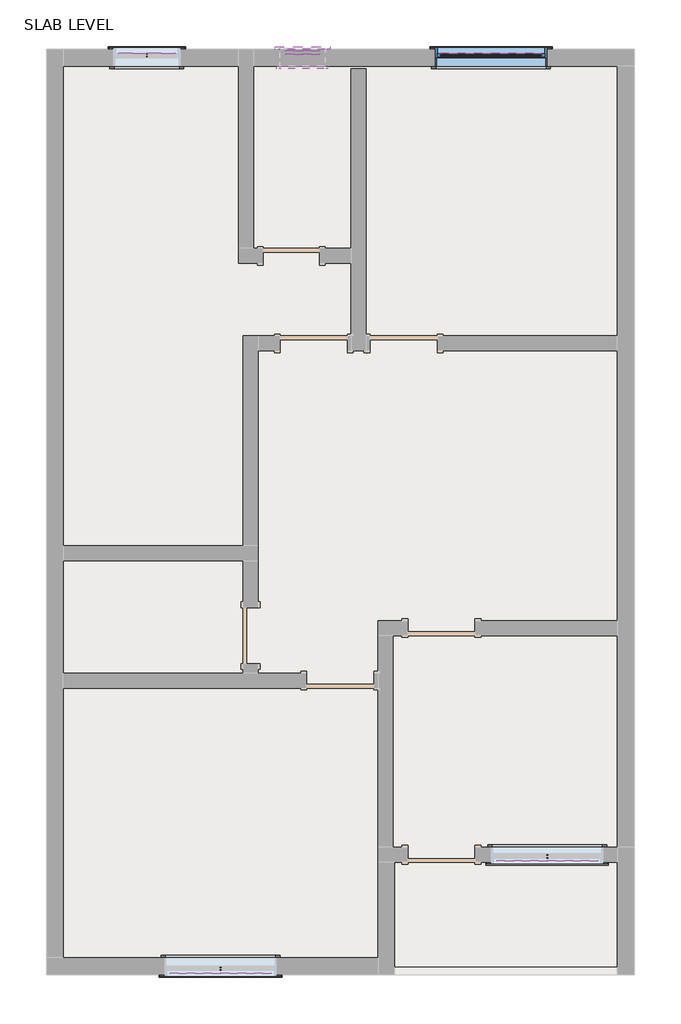
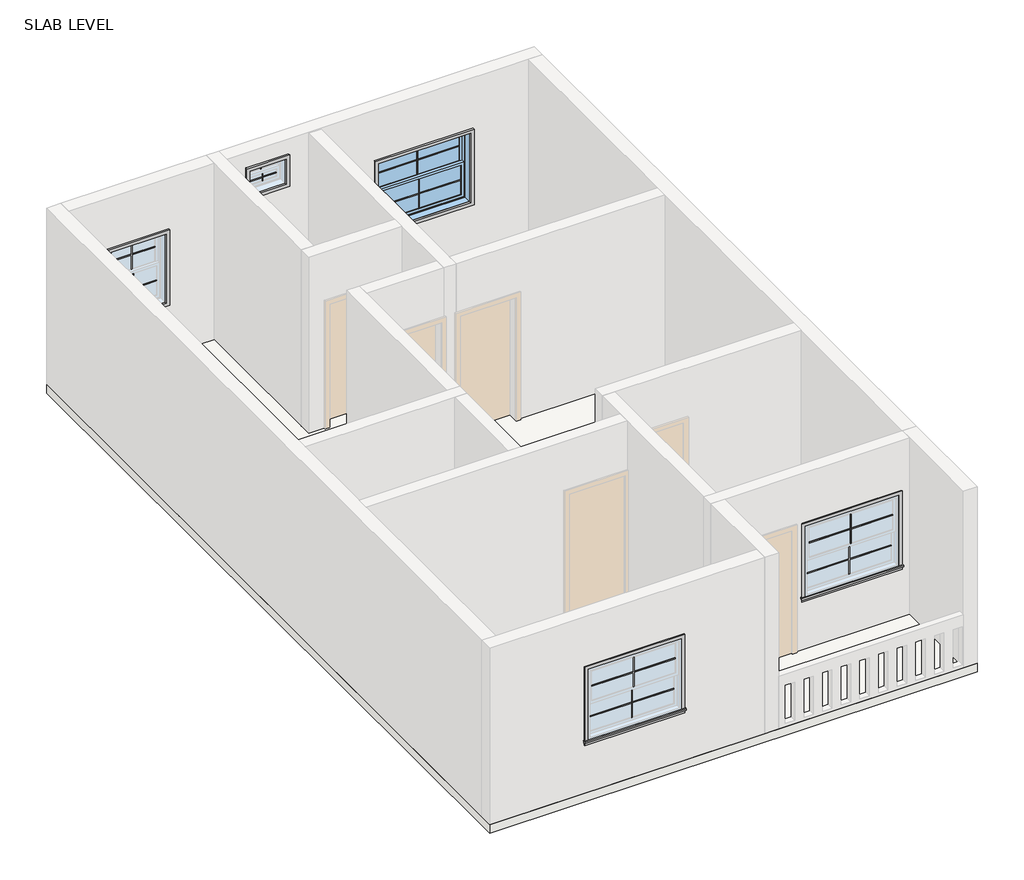
# One storey, part 2 of 2: 20 proxies, 1 railing, 1 slab, 1 window.
"""IFC4 building model written with IfcOpenShell, lengths in millimetres."""

from ifc_helpers import new_model, si_unit, frame, origin, place, context, project, spatial, polyline, outline, extrude, faceted_brep, transform, mapped, element, save
from components import muntin_pattern_2x2_muntin_pattern_2x2_c001a7f4, muntin_pattern_2x2_muntin_pattern_2x2_019d64ce, muntin_pattern_2x2_muntin_pattern_2x2_f2410a90, trim_window_exterior_flat_with_sill_7631c5ba, trim_window_exterior_flat_with_sill_f6d2a3b8, trim_window_exterior_flat_with_sill_e4b28ec3, trim_window_interior_flat_picture_frame_0f2e31f9, trim_window_interior_flat_picture_frame_f985c0ae, trim_window_interior_flat_picture_frame_39ff4276, window_a144fa31

model = new_model("IFC4")

# Units and contexts
model_context = context("Model", 3, world=origin())
ifc_project = project(units=[si_unit("LENGTHUNIT", "METRE", prefix="MILLI")], contexts=[model_context])

# Site, building, storey
site = spatial("IfcSite", under=ifc_project)
building = spatial("IfcBuilding", under=site)
storey = spatial("IfcBuildingStorey", under=building, Name="SLAB LEVEL", Elevation=3048.0)

# Proxies
placement = place(None, origin())
muntin_pattern_2x2_muntin_pattern_2x2_shape = muntin_pattern_2x2_muntin_pattern_2x2_c001a7f4(model_context)
element("IfcBuildingElementProxy", 1, Name="Muntin Pattern_2x2 : Muntin Pattern_2x2", ObjectType="Muntin Pattern_2x2 : Muntin Pattern_2x2", at=placement, inside=storey, context=model_context, shape_type="MappedRepresentation", body=[
    mapped(muntin_pattern_2x2_muntin_pattern_2x2_shape, transform((-1687.6519453, 5530.9694012, 4594.225), x_axis=(-1.0, 0.0, 0.0), y_axis=(0.0, -1.0, 0.0), z_axis=(0.0, 0.0, 1.0))),
])
element("IfcBuildingElementProxy", 2, Name="Muntin Pattern_2x2 : Muntin Pattern_2x2", ObjectType="Muntin Pattern_2x2 : Muntin Pattern_2x2", at=placement, inside=storey, context=model_context, shape_type="MappedRepresentation", body=[
    mapped(muntin_pattern_2x2_muntin_pattern_2x2_shape, transform((-1687.6519453, 5575.4194012, 4038.6), x_axis=(-1.0, 0.0, 0.0), y_axis=(0.0, -1.0, 0.0), z_axis=(0.0, 0.0, 1.0))),
])
element("IfcBuildingElementProxy", 3, Name="Muntin Pattern_2x2 : Muntin Pattern_2x2", ObjectType="Muntin Pattern_2x2 : Muntin Pattern_2x2", at=placement, inside=storey, context=model_context, shape_type="MappedRepresentation", body=[
    mapped(muntin_pattern_2x2_muntin_pattern_2x2_shape, transform((-6119.9519453, 4006.9694012, 4594.225), x_axis=(-1.0, 0.0, 0.0), y_axis=(0.0, -1.0, 0.0), z_axis=(0.0, 0.0, 1.0))),
])
element("IfcBuildingElementProxy", 4, Name="Muntin Pattern_2x2 : Muntin Pattern_2x2", ObjectType="Muntin Pattern_2x2 : Muntin Pattern_2x2", at=placement, inside=storey, context=model_context, shape_type="MappedRepresentation", body=[
    mapped(muntin_pattern_2x2_muntin_pattern_2x2_shape, transform((-6119.9519453, 4051.4194012, 4038.6), x_axis=(-1.0, 0.0, 0.0), y_axis=(0.0, -1.0, 0.0), z_axis=(0.0, 0.0, 1.0))),
])
element("IfcBuildingElementProxy", 5, Name="Muntin Pattern_2x2 : Muntin Pattern_2x2", ObjectType="Muntin Pattern_2x2 : Muntin Pattern_2x2", at=placement, inside=storey, context=model_context, shape_type="MappedRepresentation", body=[
    mapped(muntin_pattern_2x2_muntin_pattern_2x2_shape, transform((-2449.6519453, 16484.7194012, 4594.225), x_axis=(1.0, 0.0, 0.0), y_axis=(0.0, 1.0, 0.0), z_axis=(0.0, 0.0, 1.0))),
])
element("IfcBuildingElementProxy", 6, Name="Muntin Pattern_2x2 : Muntin Pattern_2x2", ObjectType="Muntin Pattern_2x2 : Muntin Pattern_2x2", at=placement, inside=storey, context=model_context, shape_type="MappedRepresentation", body=[
    mapped(muntin_pattern_2x2_muntin_pattern_2x2_shape, transform((-2449.6519453, 16440.2694012, 4038.6), x_axis=(1.0, 0.0, 0.0), y_axis=(0.0, 1.0, 0.0), z_axis=(0.0, 0.0, 1.0))),
])
muntin_pattern_2x2_muntin_pattern_2x2_2_shape = muntin_pattern_2x2_muntin_pattern_2x2_019d64ce(model_context)
element("IfcBuildingElementProxy", 7, Name="Muntin Pattern_2x2 : Muntin Pattern_2x2", ObjectType="Muntin Pattern_2x2 : Muntin Pattern_2x2", at=placement, inside=storey, context=model_context, shape_type="MappedRepresentation", body=[
    mapped(muntin_pattern_2x2_muntin_pattern_2x2_2_shape, transform((-5008.7019453, 16484.7194012, 5584.825), x_axis=(1.0, 0.0, 0.0), y_axis=(0.0, 1.0, 0.0), z_axis=(0.0, 0.0, 1.0))),
])
element("IfcBuildingElementProxy", 8, Name="Muntin Pattern_2x2 : Muntin Pattern_2x2", ObjectType="Muntin Pattern_2x2 : Muntin Pattern_2x2", at=placement, inside=storey, context=model_context, shape_type="MappedRepresentation", body=[
    mapped(muntin_pattern_2x2_muntin_pattern_2x2_2_shape, transform((-5008.7019453, 16440.2694012, 5410.2), x_axis=(1.0, 0.0, 0.0), y_axis=(0.0, 1.0, 0.0), z_axis=(0.0, 0.0, 1.0))),
])
muntin_pattern_2x2_muntin_pattern_2x2_3_shape = muntin_pattern_2x2_muntin_pattern_2x2_f2410a90(model_context)
element("IfcBuildingElementProxy", 9, Name="Muntin Pattern_2x2 : Muntin Pattern_2x2", ObjectType="Muntin Pattern_2x2 : Muntin Pattern_2x2", at=placement, inside=storey, context=model_context, shape_type="MappedRepresentation", body=[
    mapped(muntin_pattern_2x2_muntin_pattern_2x2_3_shape, transform((-7120.0769453, 16484.7194012, 4594.225), x_axis=(1.0, 0.0, 0.0), y_axis=(0.0, 1.0, 0.0), z_axis=(0.0, 0.0, 1.0))),
])
element("IfcBuildingElementProxy", 10, Name="Muntin Pattern_2x2 : Muntin Pattern_2x2", ObjectType="Muntin Pattern_2x2 : Muntin Pattern_2x2", at=placement, inside=storey, context=model_context, shape_type="MappedRepresentation", body=[
    mapped(muntin_pattern_2x2_muntin_pattern_2x2_3_shape, transform((-7120.0769453, 16440.2694012, 4038.6), x_axis=(1.0, 0.0, 0.0), y_axis=(0.0, 1.0, 0.0), z_axis=(0.0, 0.0, 1.0))),
])
trim_window_exterior_flat_with_sill_shape = trim_window_exterior_flat_with_sill_7631c5ba(model_context)
element("IfcBuildingElementProxy", 11, Name="Trim-Window-Exterior-Flat : with Sill", ObjectType="Trim-Window-Exterior-Flat : with Sill", at=placement, inside=storey, context=model_context, shape_type="MappedRepresentation", body=[
    mapped(trim_window_exterior_flat_with_sill_shape, transform((-1687.6519453, 5496.0444012, 5181.6), x_axis=(1.0, 0.0, 0.0), y_axis=(0.0, 0.0, 1.0), z_axis=(0.0, -1.0, 0.0))),
])
element("IfcBuildingElementProxy", 12, Name="Trim-Window-Exterior-Flat : with Sill", ObjectType="Trim-Window-Exterior-Flat : with Sill", at=placement, inside=storey, context=model_context, shape_type="MappedRepresentation", body=[
    mapped(trim_window_exterior_flat_with_sill_shape, transform((-6119.9519453, 3972.0444012, 5181.6), x_axis=(1.0, 0.0, 0.0), y_axis=(0.0, 0.0, 1.0), z_axis=(0.0, -1.0, 0.0))),
])
element("IfcBuildingElementProxy", 13, Name="Trim-Window-Exterior-Flat : with Sill", ObjectType="Trim-Window-Exterior-Flat : with Sill", at=placement, inside=storey, context=model_context, shape_type="MappedRepresentation", body=[
    mapped(trim_window_exterior_flat_with_sill_shape, transform((-2449.6519453, 16519.6444012, 5181.6), x_axis=(-1.0, 0.0, 0.0), y_axis=(0.0, 0.0, 1.0), z_axis=(0.0, 1.0, 0.0))),
])
trim_window_exterior_flat_with_sill_2_shape = trim_window_exterior_flat_with_sill_f6d2a3b8(model_context)
element("IfcBuildingElementProxy", 14, Name="Trim-Window-Exterior-Flat : with Sill", ObjectType="Trim-Window-Exterior-Flat : with Sill", at=placement, inside=storey, context=model_context, shape_type="MappedRepresentation", body=[
    mapped(trim_window_exterior_flat_with_sill_2_shape, transform((-5008.7019453, 16519.6444012, 5791.2), x_axis=(-1.0, 0.0, 0.0), y_axis=(0.0, 0.0, 1.0), z_axis=(0.0, 1.0, 0.0))),
])
trim_window_exterior_flat_with_sill_3_shape = trim_window_exterior_flat_with_sill_e4b28ec3(model_context)
element("IfcBuildingElementProxy", 15, Name="Trim-Window-Exterior-Flat : with Sill", ObjectType="Trim-Window-Exterior-Flat : with Sill", at=placement, inside=storey, context=model_context, shape_type="MappedRepresentation", body=[
    mapped(trim_window_exterior_flat_with_sill_3_shape, transform((-7120.0769453, 16519.6444012, 5181.6), x_axis=(-1.0, 0.0, 0.0), y_axis=(0.0, 0.0, 1.0), z_axis=(0.0, 1.0, 0.0))),
])
trim_window_interior_flat_picture_frame_shape = trim_window_interior_flat_picture_frame_0f2e31f9(model_context)
element("IfcBuildingElementProxy", 16, Name="Trim-Window-Interior-Flat : Picture Frame", ObjectType="Trim-Window-Interior-Flat : Picture Frame", at=placement, inside=storey, context=model_context, shape_type="MappedRepresentation", body=[
    mapped(trim_window_interior_flat_picture_frame_shape, transform((-1687.6519453, 5699.2444012, 5181.6), x_axis=(-1.0, 0.0, 0.0), y_axis=(0.0, 0.0, 1.0), z_axis=(0.0, 1.0, 0.0))),
])
element("IfcBuildingElementProxy", 17, Name="Trim-Window-Interior-Flat : Picture Frame", ObjectType="Trim-Window-Interior-Flat : Picture Frame", at=placement, inside=storey, context=model_context, shape_type="MappedRepresentation", body=[
    mapped(trim_window_interior_flat_picture_frame_shape, transform((-6119.9519453, 4200.6444012, 5181.6), x_axis=(-1.0, 0.0, 0.0), y_axis=(0.0, 0.0, 1.0), z_axis=(0.0, 1.0, 0.0))),
])
element("IfcBuildingElementProxy", 18, Name="Trim-Window-Interior-Flat : Picture Frame", ObjectType="Trim-Window-Interior-Flat : Picture Frame", at=placement, inside=storey, context=model_context, shape_type="MappedRepresentation", body=[
    mapped(trim_window_interior_flat_picture_frame_shape, transform((-2449.6519453, 16291.0444012, 5181.6), x_axis=(1.0, 0.0, 0.0), y_axis=(0.0, 0.0, 1.0), z_axis=(0.0, -1.0, 0.0))),
])
trim_window_interior_flat_picture_frame_2_shape = trim_window_interior_flat_picture_frame_f985c0ae(model_context)
element("IfcBuildingElementProxy", 19, Name="Trim-Window-Interior-Flat : Picture Frame", ObjectType="Trim-Window-Interior-Flat : Picture Frame", at=placement, inside=storey, context=model_context, shape_type="MappedRepresentation", body=[
    mapped(trim_window_interior_flat_picture_frame_2_shape, transform((-5008.7019453, 16291.0444012, 5791.2), x_axis=(1.0, 0.0, 0.0), y_axis=(0.0, 0.0, 1.0), z_axis=(0.0, -1.0, 0.0))),
])
trim_window_interior_flat_picture_frame_3_shape = trim_window_interior_flat_picture_frame_39ff4276(model_context)
element("IfcBuildingElementProxy", 20, Name="Trim-Window-Interior-Flat : Picture Frame", ObjectType="Trim-Window-Interior-Flat : Picture Frame", at=placement, inside=storey, context=model_context, shape_type="MappedRepresentation", body=[
    mapped(trim_window_interior_flat_picture_frame_3_shape, transform((-7120.0769453, 16291.0444012, 5181.6), x_axis=(1.0, 0.0, 0.0), y_axis=(0.0, 0.0, 1.0), z_axis=(0.0, -1.0, 0.0))),
])

# Railing
element("IfcRailing", 21, ObjectType="Handrail - Rectangular", at=placement, inside=storey, context=model_context, shape_type="SolidModel", body=[
    faceted_brep([(-3275.1519453, 16430.7444012, 1828.8), (-3275.1519453, 16430.7444012, 1778.0), (-3275.1519453, 16379.9444012, 1778.0), (-3275.1519453, 16379.9444012, 1828.8), (-595.4519453, 16430.7444012, 1828.8), (-595.4519453, 16430.7444012, 1778.0), (-646.2519453, 16379.9444012, 1778.0), (-646.2519453, 16379.9444012, 1828.8), (-595.4519453, 14970.2444012, 1828.8), (-646.2519453, 14970.2444012, 1828.8), (-646.2519453, 14970.2444012, 1778.0), (-595.4519453, 14970.2444012, 1778.0)], [[[0, 1, 2, 3]], [[1, 0, 4, 5]], [[2, 1, 5, 6]], [[3, 2, 6, 7]], [[0, 3, 7, 4]], [[8, 9, 10, 11]], [[5, 4, 8, 11]], [[6, 5, 11, 10]], [[7, 6, 10, 9]], [[4, 7, 9, 8]]]),
    extrude(outline(polyline([(-630.3769453, 14992.4694012), (-611.3269453, 14992.4694012), (-611.3269453, 14973.4194012), (-630.3769453, 14973.4194012), (-630.3769453, 14992.4694012)])), frame((0.0, 0.0, 914.4), z_axis=(0.0, 0.0, 1.0), x_axis=(1.0, 0.0, 0.0)), (0.0, 0.0, 1.0), 863.6),
    extrude(outline(polyline([(-630.3769453, 15094.0694012), (-611.3269453, 15094.0694012), (-611.3269453, 15075.0194012), (-630.3769453, 15075.0194012), (-630.3769453, 15094.0694012)])), frame((0.0, 0.0, 914.4), z_axis=(0.0, 0.0, 1.0), x_axis=(1.0, 0.0, 0.0)), (0.0, 0.0, 1.0), 863.6),
    extrude(outline(polyline([(-630.3769453, 15195.6694012), (-611.3269453, 15195.6694012), (-611.3269453, 15176.6194012), (-630.3769453, 15176.6194012), (-630.3769453, 15195.6694012)])), frame((0.0, 0.0, 914.4), z_axis=(0.0, 0.0, 1.0), x_axis=(1.0, 0.0, 0.0)), (0.0, 0.0, 1.0), 863.6),
    extrude(outline(polyline([(-630.3769453, 15297.2694012), (-611.3269453, 15297.2694012), (-611.3269453, 15278.2194012), (-630.3769453, 15278.2194012), (-630.3769453, 15297.2694012)])), frame((0.0, 0.0, 914.4), z_axis=(0.0, 0.0, 1.0), x_axis=(1.0, 0.0, 0.0)), (0.0, 0.0, 1.0), 863.6),
    extrude(outline(polyline([(-630.3769453, 15398.8694012), (-611.3269453, 15398.8694012), (-611.3269453, 15379.8194012), (-630.3769453, 15379.8194012), (-630.3769453, 15398.8694012)])), frame((0.0, 0.0, 914.4), z_axis=(0.0, 0.0, 1.0), x_axis=(1.0, 0.0, 0.0)), (0.0, 0.0, 1.0), 863.6),
    extrude(outline(polyline([(-630.3769453, 15500.4694012), (-611.3269453, 15500.4694012), (-611.3269453, 15481.4194012), (-630.3769453, 15481.4194012), (-630.3769453, 15500.4694012)])), frame((0.0, 0.0, 914.4), z_axis=(0.0, 0.0, 1.0), x_axis=(1.0, 0.0, 0.0)), (0.0, 0.0, 1.0), 863.6),
    extrude(outline(polyline([(-630.3769453, 15602.0694012), (-611.3269453, 15602.0694012), (-611.3269453, 15583.0194012), (-630.3769453, 15583.0194012), (-630.3769453, 15602.0694012)])), frame((0.0, 0.0, 914.4), z_axis=(0.0, 0.0, 1.0), x_axis=(1.0, 0.0, 0.0)), (0.0, 0.0, 1.0), 863.6),
    extrude(outline(polyline([(-630.3769453, 15703.6694012), (-611.3269453, 15703.6694012), (-611.3269453, 15684.6194012), (-630.3769453, 15684.6194012), (-630.3769453, 15703.6694012)])), frame((0.0, 0.0, 914.4), z_axis=(0.0, 0.0, 1.0), x_axis=(1.0, 0.0, 0.0)), (0.0, 0.0, 1.0), 863.6),
    extrude(outline(polyline([(-630.3769453, 15805.2694012), (-611.3269453, 15805.2694012), (-611.3269453, 15786.2194012), (-630.3769453, 15786.2194012), (-630.3769453, 15805.2694012)])), frame((0.0, 0.0, 914.4), z_axis=(0.0, 0.0, 1.0), x_axis=(1.0, 0.0, 0.0)), (0.0, 0.0, 1.0), 863.6),
    extrude(outline(polyline([(-630.3769453, 15906.8694012), (-611.3269453, 15906.8694012), (-611.3269453, 15887.8194012), (-630.3769453, 15887.8194012), (-630.3769453, 15906.8694012)])), frame((0.0, 0.0, 914.4), z_axis=(0.0, 0.0, 1.0), x_axis=(1.0, 0.0, 0.0)), (0.0, 0.0, 1.0), 863.6),
    extrude(outline(polyline([(-630.3769453, 16008.4694012), (-611.3269453, 16008.4694012), (-611.3269453, 15989.4194012), (-630.3769453, 15989.4194012), (-630.3769453, 16008.4694012)])), frame((0.0, 0.0, 914.4), z_axis=(0.0, 0.0, 1.0), x_axis=(1.0, 0.0, 0.0)), (0.0, 0.0, 1.0), 863.6),
    extrude(outline(polyline([(-630.3769453, 16110.0694012), (-611.3269453, 16110.0694012), (-611.3269453, 16091.0194012), (-630.3769453, 16091.0194012), (-630.3769453, 16110.0694012)])), frame((0.0, 0.0, 914.4), z_axis=(0.0, 0.0, 1.0), x_axis=(1.0, 0.0, 0.0)), (0.0, 0.0, 1.0), 863.6),
    extrude(outline(polyline([(-630.3769453, 16211.6694012), (-611.3269453, 16211.6694012), (-611.3269453, 16192.6194012), (-630.3769453, 16192.6194012), (-630.3769453, 16211.6694012)])), frame((0.0, 0.0, 914.4), z_axis=(0.0, 0.0, 1.0), x_axis=(1.0, 0.0, 0.0)), (0.0, 0.0, 1.0), 863.6),
    extrude(outline(polyline([(-630.3769453, 16313.2694012), (-611.3269453, 16313.2694012), (-611.3269453, 16294.2194012), (-630.3769453, 16294.2194012), (-630.3769453, 16313.2694012)])), frame((0.0, 0.0, 914.4), z_axis=(0.0, 0.0, 1.0), x_axis=(1.0, 0.0, 0.0)), (0.0, 0.0, 1.0), 863.6),
    extrude(outline(polyline([(-643.0769453, 16395.8194012), (-643.0769453, 16414.8694012), (-624.0269453, 16414.8694012), (-624.0269453, 16395.8194012), (-643.0769453, 16395.8194012)])), frame((0.0, 0.0, 914.4), z_axis=(0.0, 0.0, 1.0), x_axis=(1.0, 0.0, 0.0)), (0.0, 0.0, 1.0), 863.6),
    extrude(outline(polyline([(-744.6769453, 16395.8194012), (-744.6769453, 16414.8694012), (-725.6269453, 16414.8694012), (-725.6269453, 16395.8194012), (-744.6769453, 16395.8194012)])), frame((0.0, 0.0, 914.4), z_axis=(0.0, 0.0, 1.0), x_axis=(1.0, 0.0, 0.0)), (0.0, 0.0, 1.0), 863.6),
    extrude(outline(polyline([(-846.2769453, 16395.8194012), (-846.2769453, 16414.8694012), (-827.2269453, 16414.8694012), (-827.2269453, 16395.8194012), (-846.2769453, 16395.8194012)])), frame((0.0, 0.0, 914.4), z_axis=(0.0, 0.0, 1.0), x_axis=(1.0, 0.0, 0.0)), (0.0, 0.0, 1.0), 863.6),
    extrude(outline(polyline([(-947.8769453, 16395.8194012), (-947.8769453, 16414.8694012), (-928.8269453, 16414.8694012), (-928.8269453, 16395.8194012), (-947.8769453, 16395.8194012)])), frame((0.0, 0.0, 914.4), z_axis=(0.0, 0.0, 1.0), x_axis=(1.0, 0.0, 0.0)), (0.0, 0.0, 1.0), 863.6),
    extrude(outline(polyline([(-1049.4769453, 16395.8194012), (-1049.4769453, 16414.8694012), (-1030.4269453, 16414.8694012), (-1030.4269453, 16395.8194012), (-1049.4769453, 16395.8194012)])), frame((0.0, 0.0, 914.4), z_axis=(0.0, 0.0, 1.0), x_axis=(1.0, 0.0, 0.0)), (0.0, 0.0, 1.0), 863.6),
    extrude(outline(polyline([(-1151.0769453, 16395.8194012), (-1151.0769453, 16414.8694012), (-1132.0269453, 16414.8694012), (-1132.0269453, 16395.8194012), (-1151.0769453, 16395.8194012)])), frame((0.0, 0.0, 914.4), z_axis=(0.0, 0.0, 1.0), x_axis=(1.0, 0.0, 0.0)), (0.0, 0.0, 1.0), 863.6),
    extrude(outline(polyline([(-1252.6769453, 16395.8194012), (-1252.6769453, 16414.8694012), (-1233.6269453, 16414.8694012), (-1233.6269453, 16395.8194012), (-1252.6769453, 16395.8194012)])), frame((0.0, 0.0, 914.4), z_axis=(0.0, 0.0, 1.0), x_axis=(1.0, 0.0, 0.0)), (0.0, 0.0, 1.0), 863.6),
    extrude(outline(polyline([(-1354.2769453, 16395.8194012), (-1354.2769453, 16414.8694012), (-1335.2269453, 16414.8694012), (-1335.2269453, 16395.8194012), (-1354.2769453, 16395.8194012)])), frame((0.0, 0.0, 914.4), z_axis=(0.0, 0.0, 1.0), x_axis=(1.0, 0.0, 0.0)), (0.0, 0.0, 1.0), 863.6),
    extrude(outline(polyline([(-1455.8769453, 16395.8194012), (-1455.8769453, 16414.8694012), (-1436.8269453, 16414.8694012), (-1436.8269453, 16395.8194012), (-1455.8769453, 16395.8194012)])), frame((0.0, 0.0, 914.4), z_axis=(0.0, 0.0, 1.0), x_axis=(1.0, 0.0, 0.0)), (0.0, 0.0, 1.0), 863.6),
    extrude(outline(polyline([(-1557.4769453, 16395.8194012), (-1557.4769453, 16414.8694012), (-1538.4269453, 16414.8694012), (-1538.4269453, 16395.8194012), (-1557.4769453, 16395.8194012)])), frame((0.0, 0.0, 914.4), z_axis=(0.0, 0.0, 1.0), x_axis=(1.0, 0.0, 0.0)), (0.0, 0.0, 1.0), 863.6),
    extrude(outline(polyline([(-1659.0769453, 16395.8194012), (-1659.0769453, 16414.8694012), (-1640.0269453, 16414.8694012), (-1640.0269453, 16395.8194012), (-1659.0769453, 16395.8194012)])), frame((0.0, 0.0, 914.4), z_axis=(0.0, 0.0, 1.0), x_axis=(1.0, 0.0, 0.0)), (0.0, 0.0, 1.0), 863.6),
    extrude(outline(polyline([(-1760.6769453, 16395.8194012), (-1760.6769453, 16414.8694012), (-1741.6269453, 16414.8694012), (-1741.6269453, 16395.8194012), (-1760.6769453, 16395.8194012)])), frame((0.0, 0.0, 914.4), z_axis=(0.0, 0.0, 1.0), x_axis=(1.0, 0.0, 0.0)), (0.0, 0.0, 1.0), 863.6),
    extrude(outline(polyline([(-1862.2769453, 16395.8194012), (-1862.2769453, 16414.8694012), (-1843.2269453, 16414.8694012), (-1843.2269453, 16395.8194012), (-1862.2769453, 16395.8194012)])), frame((0.0, 0.0, 914.4), z_axis=(0.0, 0.0, 1.0), x_axis=(1.0, 0.0, 0.0)), (0.0, 0.0, 1.0), 863.6),
    extrude(outline(polyline([(-1963.8769453, 16395.8194012), (-1963.8769453, 16414.8694012), (-1944.8269453, 16414.8694012), (-1944.8269453, 16395.8194012), (-1963.8769453, 16395.8194012)])), frame((0.0, 0.0, 914.4), z_axis=(0.0, 0.0, 1.0), x_axis=(1.0, 0.0, 0.0)), (0.0, 0.0, 1.0), 863.6),
    extrude(outline(polyline([(-2065.4769453, 16395.8194012), (-2065.4769453, 16414.8694012), (-2046.4269453, 16414.8694012), (-2046.4269453, 16395.8194012), (-2065.4769453, 16395.8194012)])), frame((0.0, 0.0, 914.4), z_axis=(0.0, 0.0, 1.0), x_axis=(1.0, 0.0, 0.0)), (0.0, 0.0, 1.0), 863.6),
    extrude(outline(polyline([(-2167.0769453, 16395.8194012), (-2167.0769453, 16414.8694012), (-2148.0269453, 16414.8694012), (-2148.0269453, 16395.8194012), (-2167.0769453, 16395.8194012)])), frame((0.0, 0.0, 914.4), z_axis=(0.0, 0.0, 1.0), x_axis=(1.0, 0.0, 0.0)), (0.0, 0.0, 1.0), 863.6),
    extrude(outline(polyline([(-2268.6769453, 16395.8194012), (-2268.6769453, 16414.8694012), (-2249.6269453, 16414.8694012), (-2249.6269453, 16395.8194012), (-2268.6769453, 16395.8194012)])), frame((0.0, 0.0, 914.4), z_axis=(0.0, 0.0, 1.0), x_axis=(1.0, 0.0, 0.0)), (0.0, 0.0, 1.0), 863.6),
    extrude(outline(polyline([(-2370.2769453, 16395.8194012), (-2370.2769453, 16414.8694012), (-2351.2269453, 16414.8694012), (-2351.2269453, 16395.8194012), (-2370.2769453, 16395.8194012)])), frame((0.0, 0.0, 914.4), z_axis=(0.0, 0.0, 1.0), x_axis=(1.0, 0.0, 0.0)), (0.0, 0.0, 1.0), 863.6),
    extrude(outline(polyline([(-2471.8769453, 16395.8194012), (-2471.8769453, 16414.8694012), (-2452.8269453, 16414.8694012), (-2452.8269453, 16395.8194012), (-2471.8769453, 16395.8194012)])), frame((0.0, 0.0, 914.4), z_axis=(0.0, 0.0, 1.0), x_axis=(1.0, 0.0, 0.0)), (0.0, 0.0, 1.0), 863.6),
    extrude(outline(polyline([(-2573.4769453, 16395.8194012), (-2573.4769453, 16414.8694012), (-2554.4269453, 16414.8694012), (-2554.4269453, 16395.8194012), (-2573.4769453, 16395.8194012)])), frame((0.0, 0.0, 914.4), z_axis=(0.0, 0.0, 1.0), x_axis=(1.0, 0.0, 0.0)), (0.0, 0.0, 1.0), 863.6),
    extrude(outline(polyline([(-2675.0769453, 16395.8194012), (-2675.0769453, 16414.8694012), (-2656.0269453, 16414.8694012), (-2656.0269453, 16395.8194012), (-2675.0769453, 16395.8194012)])), frame((0.0, 0.0, 914.4), z_axis=(0.0, 0.0, 1.0), x_axis=(1.0, 0.0, 0.0)), (0.0, 0.0, 1.0), 863.6),
    extrude(outline(polyline([(-2776.6769453, 16395.8194012), (-2776.6769453, 16414.8694012), (-2757.6269453, 16414.8694012), (-2757.6269453, 16395.8194012), (-2776.6769453, 16395.8194012)])), frame((0.0, 0.0, 914.4), z_axis=(0.0, 0.0, 1.0), x_axis=(1.0, 0.0, 0.0)), (0.0, 0.0, 1.0), 863.6),
    extrude(outline(polyline([(-2878.2769453, 16395.8194012), (-2878.2769453, 16414.8694012), (-2859.2269453, 16414.8694012), (-2859.2269453, 16395.8194012), (-2878.2769453, 16395.8194012)])), frame((0.0, 0.0, 914.4), z_axis=(0.0, 0.0, 1.0), x_axis=(1.0, 0.0, 0.0)), (0.0, 0.0, 1.0), 863.6),
    extrude(outline(polyline([(-2979.8769453, 16395.8194012), (-2979.8769453, 16414.8694012), (-2960.8269453, 16414.8694012), (-2960.8269453, 16395.8194012), (-2979.8769453, 16395.8194012)])), frame((0.0, 0.0, 914.4), z_axis=(0.0, 0.0, 1.0), x_axis=(1.0, 0.0, 0.0)), (0.0, 0.0, 1.0), 863.6),
    extrude(outline(polyline([(-3081.4769453, 16395.8194012), (-3081.4769453, 16414.8694012), (-3062.4269453, 16414.8694012), (-3062.4269453, 16395.8194012), (-3081.4769453, 16395.8194012)])), frame((0.0, 0.0, 914.4), z_axis=(0.0, 0.0, 1.0), x_axis=(1.0, 0.0, 0.0)), (0.0, 0.0, 1.0), 863.6),
    extrude(outline(polyline([(-3183.0769453, 16395.8194012), (-3183.0769453, 16414.8694012), (-3164.0269453, 16414.8694012), (-3164.0269453, 16395.8194012), (-3183.0769453, 16395.8194012)])), frame((0.0, 0.0, 914.4), z_axis=(0.0, 0.0, 1.0), x_axis=(1.0, 0.0, 0.0)), (0.0, 0.0, 1.0), 863.6),
    extrude(outline(polyline([(-630.3769453, 16395.8194012), (-630.3769453, 16414.8694012), (-611.3269453, 16414.8694012), (-611.3269453, 16395.8194012), (-630.3769453, 16395.8194012)])), frame((0.0, 0.0, 914.4), z_axis=(0.0, 0.0, 1.0), x_axis=(1.0, 0.0, 0.0)), (0.0, 0.0, 1.0), 863.6),
    extrude(outline(polyline([(-630.3769453, 14989.2944012), (-611.3269453, 14989.2944012), (-611.3269453, 14970.2444012), (-630.3769453, 14970.2444012), (-630.3769453, 14989.2944012)])), frame((0.0, 0.0, 914.4), z_axis=(0.0, 0.0, 1.0), x_axis=(1.0, 0.0, 0.0)), (0.0, 0.0, 1.0), 863.6),
    extrude(outline(polyline([(-3275.1519453, 16395.8194012), (-3275.1519453, 16414.8694012), (-3256.1019453, 16414.8694012), (-3256.1019453, 16395.8194012), (-3275.1519453, 16395.8194012)])), frame((0.0, 0.0, 914.4), z_axis=(0.0, 0.0, 1.0), x_axis=(1.0, 0.0, 0.0)), (0.0, 0.0, 1.0), 863.6),
])

# Slab
element("IfcSlab", 22, ObjectType="SLAB 6\"", at=placement, inside=storey, context=model_context, shape_type="SweptSolid", body=[
    extrude(outline(polyline([(-506.5519453, 3972.0444012), (-8482.1519453, 3972.0444012), (-8482.1519453, 16519.6444012), (-506.5519453, 16519.6444012), (-506.5519453, 3972.0444012)])), frame((0.0, 0.0, 2895.6), z_axis=(0.0, 0.0, 1.0), x_axis=(1.0, 0.0, 0.0)), (0.0, 0.0, 1.0), 152.4),
])

# Window
window_shape = window_a144fa31(model_context)
element("IfcWindow", 23, ObjectType="Window-Double-Hung : 60\"X48\"", at=placement, inside=storey, context=model_context, shape_type="MappedRepresentation", body=[
    mapped(window_shape, transform((-2449.6519453, 16405.3444012, 3048.0), x_axis=(1.0, 0.0, 0.0), y_axis=(0.0, 1.0, 0.0), z_axis=(0.0, 0.0, 1.0))),
])

save(model, "model.ifc")

# Revit data of these elements
# Type "Muntin Pattern_2x2 : Muntin Pattern_2x2"
#   Width [instance default] = 4' - 0"
#   Thickness = 0' - 0 1/2"
#   Height [instance default] = 4' - 0"
#   Distance = 0' - 0 3/4"
#   Interior Material [instance default] = none
#   Exterior Material [instance default] = none
#   Default Elevation = 0
# Type "Trim-Window-Exterior-Flat : with Sill"
#   Trim Width = 0' - 2 1/4"
#   Trim Thickness_Picture Frame = 0' - 1 1/4"
#   Trim Thickness_with Sill = 0' - 0 3/4"
#   Sill Thickness = 0' - 1 1/4"
#   Opening Width [instance default] = 2' - 0"
#   Opening Height [instance default] = 3' - 0"
#   Default Elevation = 4' - 0"
#   Sill = yes
#   Picture Frame = no
#   Trim Material [instance default] = none
# Type "Trim-Window-Interior-Flat : Picture Frame"
#   Trim Thickness_Picture Frame = 0' - 1 1/4"
#   Trim Width = 0' - 2 1/4"
#   Trim Thickness_with Sill = 0' - 0 3/4"
#   Sill Thickness = 0' - 1 1/4"
#   Opening Width [instance default] = 2' - 0"
#   Opening Height [instance default] = 3' - 0"
#   Default Elevation = 4' - 0"
#   Sill = no
#   Picture Frame = yes
#   Trim Material [instance default] = none
# Type "Handrail - Rectangular"
#   Assembly Code = "C2010400"
#   built-in parameter 1008612 = 0.0416667 (stored number, unit not read)
#   built-in parameter 1008611 = 0.0416667 (stored number, unit not read)
#   built-in parameter 1008609 = 0.333333 (stored number, unit not read)
#   built-in parameter 1008604 = 0.166667 (stored number, unit not read)
#   built-in parameter 1008603 = 0.166667 (stored number, unit not read)
#   Railing Height = 3' - 0"
#   built-in parameter 1008630 = 2
#   built-in parameter 1008610 = 2
#   built-in parameter 1008618 = Baluster - Square : 3/4"
# Type "SLAB 6\""
#   Assembly Code = "B1010"
#   Function = 0
#   Layers, outside or top first: 0' - 6" no material (function 1)
# Type "Window-Double-Hung : 60\"X48\""
#   Type Mark = "18"
#   Fire Rating = "0.5h"
#   Construction Type Id = "DG-DR"
#   Assembly Code = "B2020100"
#   Analytic Construction = "Double glazing - domestic"
#   Wall Thickness [instance default] = 0' - 6"
#   Window Inset [instance default] = 0' - 0"
#   Visual Light Transmittance = 0.81
#   Thermal Resistance (R) = 1.8146 (h·ft²·°F)/BTU
#   Solar Heat Gain Coefficient = 0.76
#   Muntin Width = 4' - 6"
#   Muntin Height = 1' - 8 1/8"
#   Interior Wall Closure [instance default] = 0' - 1 1/2"
#   Rough Width = 5' - 0 1/2"
#   Rough Height = 4' - 0 1/2"
#   Frame Extension [instance default] = 0' - 1 1/4"
#   Exterior Wall Closure [instance default] = 0' - 0 1/2"
#   Extension Jamb [instance default] = 0' - 1 1/2"
#   Heat Transfer Coefficient (U) = 0.5511 BTU/(h·ft²·°F)
#   Height = 4' - 0"
#   Width = 5' - 0"
#   Top Muntin Visibility = yes
#   Indicator Visibility [instance default] = yes
#   Extension Jamb Visibility [instance default] = yes
#   Interior Trim Visibility [instance default] = yes
#   Exterior Trim Visibility [instance default] = yes
#   Define Thermal Properties by = 1
#   Bottom Muntin Visibility = yes
#   Muntin Pattern = Muntin Pattern_2x2 : Muntin Pattern_2x2
#   Interior Trim Material = Wood - Stained
#   Interior Trim = Trim-Window-Interior-Flat : Picture Frame
#   Exterior Trim Material = Clad - White
#   Exterior Trim = Trim-Window-Exterior-Flat : with Sill
#   Glass Panel Material = Glass
#   Exterior Frame Material = Clad - White
#   Interior Frame Material = Wood - Stained
#   Wall Closure = (empty or 0)
# Elements 1, 2, 3, 4, 5, 6 (IfcBuildingElementProxy, "Muntin Pattern_2x2 : Muntin Pattern_2x2")
#   Width = 4' - 6"
#   Height = 1' - 8 1/8"
#   Interior Material = Wood - Stained
#   Exterior Material = Clad - White
#   Phase Created = New Construction
#   Materials on its faces: "Clad - White", "Wood - Stained"
# Elements 7, 8 (IfcBuildingElementProxy, "Muntin Pattern_2x2 : Muntin Pattern_2x2")
#   Width = 1' - 6"
#   Height = 0' - 5 1/8"
#   Interior Material = Wood - Stained
#   Exterior Material = Clad - White
#   Phase Created = New Construction
#   Materials on its faces: "Clad - White", "Wood - Stained"
# Elements 9, 10 (IfcBuildingElementProxy, "Muntin Pattern_2x2 : Muntin Pattern_2x2")
#   Width = 2' - 6"
#   Height = 1' - 8 1/8"
#   Interior Material = Wood - Stained
#   Exterior Material = Clad - White
#   Phase Created = New Construction
#   Materials on its faces: "Clad - White", "Wood - Stained"
# Elements 11, 12, 13 (IfcBuildingElementProxy, "Trim-Window-Exterior-Flat : with Sill")
#   Opening Width = 5' - 0"
#   Opening Height = 4' - 0"
#   Trim Material = Clad - White
#   Phase Created = New Construction
#   Materials on its faces: "Clad - White"
# Element 14 (IfcBuildingElementProxy, "Trim-Window-Exterior-Flat : with Sill")
#   Opening Width = 2' - 0"
#   Opening Height = 1' - 6"
#   Trim Material = Clad - White
#   Phase Created = New Construction
#   Materials on its faces: "Clad - White"
# Element 15 (IfcBuildingElementProxy, "Trim-Window-Exterior-Flat : with Sill")
#   Opening Width = 3' - 0"
#   Opening Height = 4' - 0"
#   Trim Material = Clad - White
#   Phase Created = New Construction
#   Materials on its faces: "Clad - White"
# Elements 16, 17, 18 (IfcBuildingElementProxy, "Trim-Window-Interior-Flat : Picture Frame")
#   Opening Width = 5' - 0"
#   Opening Height = 4' - 0"
#   Trim Material = Wood - Stained
#   Phase Created = New Construction
#   Materials on its faces: "Wood - Stained"
# Element 19 (IfcBuildingElementProxy, "Trim-Window-Interior-Flat : Picture Frame")
#   Opening Width = 2' - 0"
#   Opening Height = 1' - 6"
#   Trim Material = Wood - Stained
#   Phase Created = New Construction
#   Materials on its faces: "Wood - Stained"
# Element 20 (IfcBuildingElementProxy, "Trim-Window-Interior-Flat : Picture Frame")
#   Opening Width = 3' - 0"
#   Opening Height = 4' - 0"
#   Trim Material = Wood - Stained
#   Phase Created = New Construction
#   Materials on its faces: "Wood - Stained"
# Element 21 (IfcRailing, "Handrail - Rectangular")
#   built-in parameter 1008621 = -7 (stored number, unit not read)
#   Phase Created = New Construction
# Element 22 (IfcSlab, "SLAB 6\"")
#   built-in parameter 1001955 = -1.5708 (stored number, unit not read)
#   Height Offset From Level = 0' - 0"
#   Phase Created = New Construction
#   Materials on its faces: "Default Floor"
# Element 23 (IfcWindow, "Window-Double-Hung : 60\"X48\"")
#   Mark = "9"
#   Window Inset = 0' - 0"
#   Interior Wall Closure = 0' - 1 1/2"
#   Frame Extension = 0' - 1 1/4"
#   Exterior Wall Closure = 0' - 0 1/2"
#   Interior Trim Visibility = yes
#   Indicator Visibility = yes
#   Exterior Trim Visibility = yes
#   Phase Created = New Construction
#   Materials on its faces: "Wood - Stained", "Glass", "Clad - White"
# Materials
#   "Wood - Stained": class "Wood", colour RGB 224 178 126, transparency 0, Cost = 0
#   "Clad - White": class "Wood", colour RGB 242 242 238, transparency 0, Cost = 0
#   "Glass": class "Glass", colour RGB 0 128 192, transparency 0.75, Description = "Soda Lime Glass", Cost = 0
#   "Default Floor": colour RGB 128 128 128, transparency 0, Cost = 0
